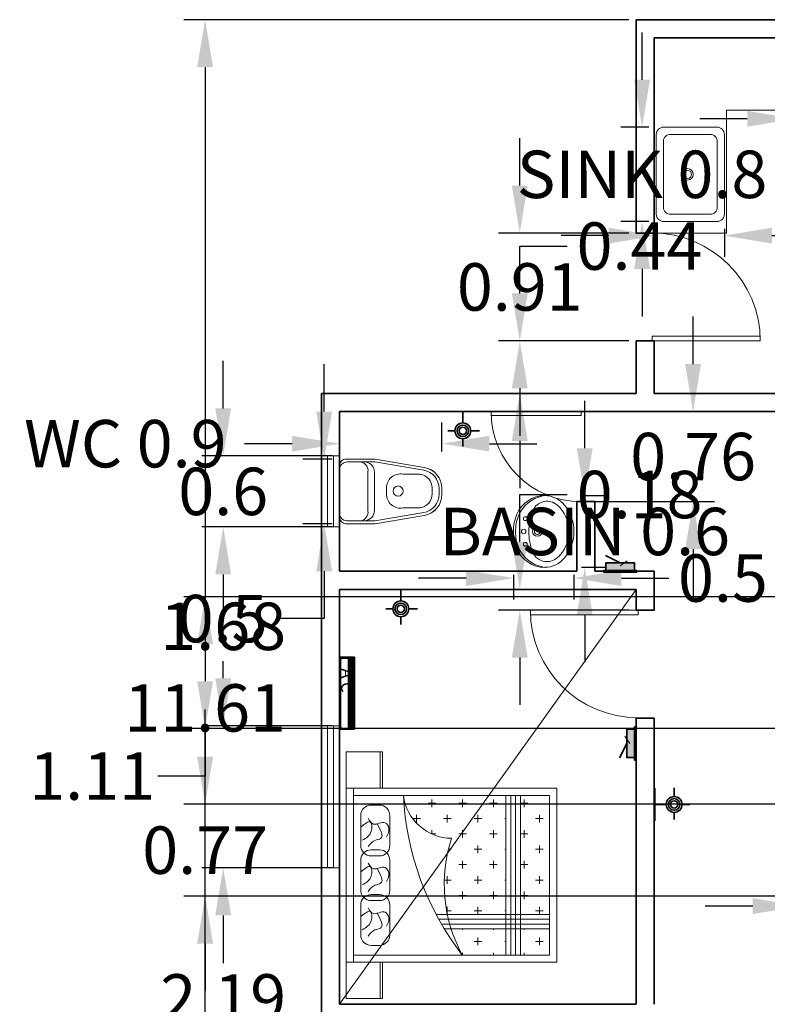
# Model space of a CAD drawing. Units: metres. Extents: x 24.2 to 58.5, y -14.5 to 15.2.
# Tile 5 of 7: x 38.9 to 45.2, y 5.2 to 13.5. Entities that reach past the tile are written whole.
import ezdxf

# ---------------------------------------------------------------- set-up
doc = ezdxf.new("R2010")
doc.units = ezdxf.units.M
doc.header["$MEASUREMENT"] = 0
for name, color, linetype, lineweight in [('A-FLOR-CASE', 163, 'Continuous', 18), ('A-FLOR-FIXT', 163, 'Continuous', 18), ('A-FURN', 150, 'Continuous', 5), ('A-GLAZ', 15, 'Continuous', 18), ('A-WALL', 7, 'Continuous', 35), ('DIMENSION', 90, 'Continuous', 18), ('DOOR', 15, 'Continuous', 18), ('E-EQPM-LAYO', 1, 'Continuous', 13), ('E-LITE', 1, 'Continuous', 18), ('E-POWR', 1, 'Continuous', 18), ('E-POWR-EQPM', 1, 'Continuous', 18), ('Elec', 1, 'Continuous', 35), ('FURN', 163, 'Continuous', 13)]:
    doc.layers.add(name, color=color, linetype=linetype, lineweight=lineweight)
doc.styles.get("Standard").update_dxf_attribs({"font": 'arial.ttf'})
doc.dimstyles.get("Standard").update_dxf_attribs({"dimtxt": 0.4, "dimasz": 0.4, "dimexe": 0.18, "dimexo": 0.0625, "dimgap": 0.09, "dimtad": 0, "dimtih": 1, "dimtoh": 1, "dimdec": 1, "dimzin": 0, "dimdsep": 46, "dimtxsty": 'Standard', "dimcen": 0.09, "dimadec": 0, "dimazin": 0, "dimtfac": 1, "dimtdec": 1, "dimtofl": 0, "dimtmove": 0, "dimatfit": 3, "dimfxl": 1, "dimtolj": 1, "dimtzin": 0, "dimarcsym": 0})

# ---------------------------------------------------------------- blocks, each defined once
blk = doc.blocks.new('*U17')
for p, q in [((0, 0), (0, -6)), ((40, 0), (40, -6))]:
    blk.add_line(p, q)
blk.add_lwpolyline([(0, 0), (0, 40), (1.75, 40), (1.75, 0)], close=True)
blk.add_arc((0, 0), 40, 0, 90)
blk = doc.blocks.new('WC')
at = {"layer": 'A-FURN'}
for p, q in [((171114.18, -56009.21), (171100.52, -56011.54)), ((171114.18, -56009.21), (171122.29, -56009.21)), ((171124.07, -56010.99), (171124.07, -56025.42)), ((171095.59, -56017.39), (171095.59, -56019.02)), ((171114.18, -56027.21), (171100.52, -56024.87)), ((171122.29, -56027.21), (171114.18, -56027.21))]:
    blk.add_line(p, q, dxfattribs=at)
for points in [[(171114.18, -56027.21), (171122.29, -56027.21, 0.414214), (171124.07, -56025.42), (171124.07, -56010.99, 0.414214), (171122.29, -56009.21), (171114.18, -56009.21), (171100.52, -56011.54, 0.365402), (171095.59, -56017.39), (171095.59, -56019.02, 0.365402), (171100.52, -56024.87)], [(171114.25, -56026.41), (171121.5, -56026.41, 0.361508), (171124.07, -56024.7), (171124.07, -56011.71, 0.375474), (171121.68, -56010), (171114.25, -56010), (171100.66, -56012.32, 0.365402), (171096.38, -56017.39), (171096.38, -56019.02, 0.365402), (171100.66, -56024.09)], [(171124.07, -56011.71), (171124.07, -56024.7, -0.361508), (171121.5, -56026.41), (171117.23, -56026.41, -0.430105), (171114.38, -56023.46), (171114.38, -56012.95, -0.411531), (171117.23, -56010), (171121.68, -56010, -0.375474)], [(171124.07, -56011.71), (171124.07, -56024.7, -0.361508), (171121.5, -56026.41), (171118.83, -56026.41, -0.480412), (171116.16, -56023.63), (171116.16, -56012.78, -0.482705), (171118.83, -56010), (171121.68, -56010, -0.375474)], [(171106.42, -56023.02, 0.46477), (171111.04, -56019.12), (171111.04, -56017.49, 0.46477), (171106.42, -56013.59), (171101.64, -56013.59, 0.365402), (171098.35, -56017.49), (171098.35, -56019.12, 0.365402), (171101.64, -56023.02)], [(171107.8, -56016.9, -1), (171107.8, -56019.71, -1)]]:
    blk.add_lwpolyline(points, format="xyb", close=True, dxfattribs=at)
for centre, radius, start, end in [((171122.29, -56010.99), 1.78, 0.0002, 90.0002), ((171101.52, -56017.39), 5.93, 99.7106, 180.0002), ((171101.52, -56019.02), 5.93, 180.0002, 260.2897), ((171122.29, -56025.42), 1.78, 270.0002, 0.0002)]:
    blk.add_arc(centre, radius, start, end, dxfattribs=at)
blk = doc.blocks.new('Basin')
at = {"layer": 'A-FURN'}
for centre, radius in [((171010.96, -56068.51), 0.593), ((171010.45, -56072.47), 0.692), ((171014.68, -56072.47), 1.48), ((171014.68, -56072.47), 0.91), ((171010.96, -56076.42), 0.593)]:
    blk.add_circle(centre, radius, dxfattribs=at)
for centre, radius, start, end in [((171018.29, -56073.43), 10.2, 262.5047, 262.5047), ((171016.96, -56070.69), 9.3, 90, 157.2856), ((171018.29, -56071.51), 10.2, 100.9967, 157.8207), ((171017.65, -56067.95), 4.81, 62.931, 159.6415), ((171016.96, -56069.3), 7.91, 39.0829, 90), ((171029.84, -56072.47), 17.8, 159.6415, 180), ((171016.96, -56069.3), 6.33, 39.0829, 62.931), ((171013.06, -56072.47), 11.35, 0, 39.0829), ((171013.06, -56072.47), 12.93, 0, 39.0829), ((171021.21, -56072.47), 13.91, 157.2856, 180), ((171021.21, -56072.47), 13.27, 158.7467, 180), ((171021.21, -56072.47), 13.91, 180, 202.7144), ((171021.21, -56072.47), 13.27, 180, 201.2533), ((171029.84, -56072.47), 17.8, 180, 200.3585), ((171013.06, -56072.47), 11.35, 320.9171, 0), ((171013.06, -56072.47), 12.93, 320.9171, 0), ((171016.96, -56074.25), 9.3, 202.7144, 270), ((171018.29, -56073.43), 10.2, 202.1793, 259.0033), ((171017.65, -56076.99), 4.81, 200.3585, 297.069), ((171016.96, -56075.63), 7.91, 270, 320.9171), ((171016.96, -56075.63), 6.33, 297.069, 320.9171)]:
    blk.add_arc(centre, radius, start, end, dxfattribs=at)
blk = doc.blocks.new('bed 1')
at = {"layer": 'FURN'}
h = blk.add_hatch(dxfattribs=at)
h.set_pattern_fill('CROSS', color=256, style=0)
h.set_pattern_definition([(0, (0, 0), (6.35, 6.35), [3.175, -9.525]), (90, (1.5875, -1.5875), (-6.35, 6.35), [3.175, -9.525])])
h.paths.add_polyline_path([(1334.16, -843.32, 0.37496), (1316.43, -863.27, 0.131129), (1284.95, -861.51), (1284.95, -885.72), (1334.16, -885.72)])
h.paths.add_polyline_path([(1278.95, -863.08, 0.048033), (1268.16, -867.67), (1268.16, -885.72), (1278.95, -885.72)])
h.paths.add_polyline_path([(1278.95, -891.72), (1268.16, -891.72), (1268.16, -903.72), (1278.95, -903.72)])
h.paths.add_polyline_path([(1334.16, -891.72), (1284.95, -891.72), (1284.95, -903.72), (1334.16, -903.72)])
for p, q in [((1265.16, -819.72), (1250.16, -819.72)), ((1250.16, -819.72), (1250.16, -834.72)), ((1337.16, -819.72), (1265.16, -819.72)), ((1265.16, -819.72), (1265.16, -906.72)), ((1337.16, -906.72), (1337.16, -819.72)), ((1337.16, -819.72), (1352.16, -819.72)), ((1352.16, -819.72), (1352.16, -834.72)), ((1337.16, -822.72), (1265.16, -822.72)), ((1268.16, -822.72), (1268.16, -903.72)), ((1334.16, -903.72), (1334.16, -822.72)), ((1250.16, -833.72), (1265.16, -833.72)), ((1352.16, -833.72), (1337.16, -833.72)), ((1250.16, -834.72), (1265.16, -834.72)), ((1352.16, -834.72), (1337.16, -834.72)), ((1282.95, -903.72), (1282.95, -857.98)), ((1284.95, -903.72), (1284.95, -856.89)), ((1278.95, -903.72), (1278.95, -860.29)), ((1280.95, -903.72), (1280.95, -859.11)), ((1334.16, -885.72), (1268.16, -885.72)), ((1334.16, -887.72), (1268.16, -887.72)), ((1334.16, -889.72), (1268.16, -889.72)), ((1334.16, -891.72), (1268.16, -891.72)), ((1268.16, -903.72), (1334.16, -903.72)), ((1265.16, -906.72), (1337.16, -906.72))]:
    blk.add_line(p, q, dxfattribs=at)
for points in [[(1288.91, -837.72), (1276.42, -837.72, -0.414214), (1272.16, -833.47), (1272.16, -829.98, -0.414214), (1276.42, -825.72), (1288.91, -825.72, -0.414214), (1293.16, -829.98), (1293.16, -833.47, -0.414214)], [(1307.41, -837.72), (1294.92, -837.72, -0.414214), (1290.66, -833.47), (1290.66, -829.98, -0.414214), (1294.92, -825.72), (1307.41, -825.72, -0.414214), (1311.66, -829.98), (1311.66, -833.47, -0.414214)], [(1325.91, -837.72), (1313.42, -837.72, -0.414214), (1309.16, -833.47), (1309.16, -829.98, -0.414214), (1313.42, -825.72), (1325.91, -825.72, -0.414214), (1330.16, -829.98), (1330.16, -833.47, -0.414214)], [(1334.16, -843.32, 0.151933), (1268.16, -867.67), (1268.16, -867.67, -0.20661), (1316.43, -863.27), (1316.43, -863.27, -0.37496)]]:
    blk.add_lwpolyline(points, format="xyb", close=True, dxfattribs=at)
for points, knots in [([(1278.62, -826.37), (1279.52, -827.92), (1281.07, -830.61), (1287.77, -830.3), (1285.41, -827.44), (1284.17, -825.93)], [0, 0, 0, 0, 4.23607, 7.317462, 10.761159, 10.761159, 10.761159, 10.761159]), ([(1297.12, -826.37), (1298.02, -827.92), (1299.57, -830.61), (1306.27, -830.3), (1303.91, -827.44), (1302.67, -825.93)], [0, 0, 0, 0, 4.23607, 7.317462, 10.761159, 10.761159, 10.761159, 10.761159]), ([(1315.62, -826.37), (1316.52, -827.92), (1318.07, -830.61), (1324.77, -830.3), (1322.41, -827.44), (1321.17, -825.93)], [0, 0, 0, 0, 4.23607, 7.317462, 10.761159, 10.761159, 10.761159, 10.761159]), ([(1275.98, -828.74), (1277, -829.54), (1278.71, -830.85), (1279.22, -835.95), (1282.92, -833.91), (1285.58, -832.44)], [0, 0, 0, 0, 3.079719, 5.108686, 10.317752, 10.317752, 10.317752, 10.317752]), ([(1287.7, -828.74), (1286.63, -829.38), (1283.96, -830.98), (1287.28, -835.52), (1283.18, -838.02), (1281.17, -836.99), (1280.03, -836.4)], [0, 0, 0, 0, 2.624379, 6.568207, 8.823918, 11.783788, 11.783788, 11.783788, 11.783788]), ([(1294.48, -828.74), (1295.5, -829.54), (1297.21, -830.85), (1297.72, -835.95), (1301.42, -833.91), (1304.08, -832.44)], [0, 0, 0, 0, 3.079719, 5.108686, 10.317752, 10.317752, 10.317752, 10.317752]), ([(1306.2, -828.74), (1305.13, -829.38), (1302.46, -830.98), (1305.78, -835.52), (1301.68, -838.02), (1299.67, -836.99), (1298.53, -836.4)], [0, 0, 0, 0, 2.624379, 6.568207, 8.823918, 11.783788, 11.783788, 11.783788, 11.783788]), ([(1312.98, -828.74), (1314, -829.54), (1315.71, -830.85), (1316.22, -835.95), (1319.92, -833.91), (1322.58, -832.44)], [0, 0, 0, 0, 3.079719, 5.108686, 10.317752, 10.317752, 10.317752, 10.317752]), ([(1324.7, -828.74), (1323.63, -829.38), (1320.96, -830.98), (1324.28, -835.52), (1320.18, -838.02), (1318.17, -836.99), (1317.03, -836.4)], [0, 0, 0, 0, 2.624379, 6.568207, 8.823918, 11.783788, 11.783788, 11.783788, 11.783788])]:
    blk.add_open_spline(points, degree=3, knots=knots, dxfattribs=at)
blk = doc.blocks.new('SINK')
at = {"layer": 'A-FURN'}
for points in [[(42.3016, 12.7524), (42.9757, 12.7524, -0.414214), (43.0363, 12.6917), (43.0363, 12.2383, -0.414214), (42.9757, 12.1776), (42.3016, 12.1776, -0.414214), (42.2409, 12.2383), (42.2409, 12.6917, -0.414214)], [(42.3622, 12.6917), (42.915, 12.6917, -0.414214), (42.9757, 12.6311), (42.9757, 12.2989, -0.414214), (42.915, 12.2383), (42.3622, 12.2383, -0.414214), (42.3016, 12.2989), (42.3016, 12.6311, -0.414214)]]:
    blk.add_lwpolyline(points, format="xyb", close=True, dxfattribs=at)
for radius in [0.0481, 0.0337]:
    blk.add_circle((42.6387, 12.4417), radius, dxfattribs=at)
blk = doc.blocks.new('splight')
at = {"layer": 'Elec'}
for p, q in [((4618.17, 527.16), (4627.57, 527.16)), ((4622.87, 527.16), (4622.87, 523.87)), ((4620.58, 521.58), (4618.05, 521.58)), ((4625.16, 521.58), (4627.23, 521.58)), ((4622.87, 519.28), (4622.87, 517.03))]:
    blk.add_line(p, q, dxfattribs=at)
for radius in [2.29, 1.67, 1.04]:
    blk.add_circle((4622.87, 521.58), radius, dxfattribs=at)
blk = doc.blocks.new('ac')
at = {"layer": 'Elec'}
for p, q in [((12718.34, -53.78), (12674.36, -53.78)), ((12674.36, -63.02), (12674.36, -53.78)), ((12675.81, -57.52), (12675.81, -53.78)), ((12717.03, -57.52), (12717.03, -53.78)), ((12718.34, -63.02), (12718.34, -53.78)), ((12674.89, -57.52), (12717.81, -57.52)), ((12717.03, -54.85), (12675.81, -54.85)), ((12717.03, -56.21), (12675.81, -56.21)), ((12718.34, -63.02), (12674.36, -63.02))]:
    blk.add_line(p, q, dxfattribs=at)
at = {"layer": 'Elec', "ltscale": 0.1}
for p, q in [((12674.89, -61.49), (12674.89, -53.78)), ((12717.81, -61.49), (12717.81, -53.78)), ((12717.03, -54.36), (12675.81, -54.36)), ((12717.03, -55.66), (12675.81, -55.66)), ((12717.03, -56.84), (12675.81, -56.84)), ((12716.81, -62.49), (12675.89, -62.49))]:
    blk.add_line(p, q, dxfattribs=at)
at = {"layer": 'Elec'}
for centre, start, end in [((12675.89, -61.49), 180, 270), ((12716.81, -61.49), 270, 0)]:
    blk.add_arc(centre, 1, start, end, dxfattribs=at)
blk = doc.blocks.new('WINDOW-1200')
for p, q in [((0.1529, 1.1998), (0.0005, 1.1998)), ((0.0513, -0.0002), (0.0513, 1.1998)), ((0.1021, -0.0002), (0.1021, 1.1998)), ((0.1529, -0.0002), (0.0005, -0.0002))]:
    blk.add_line(p, q)
blk = doc.blocks.new('elec box')
at = {"layer": 'Elec'}
blk.add_hatch(color=256, dxfattribs=at).paths.add_polyline_path([(3828.23, 599.29), (3828.23, 594.79), (3844.73, 594.79), (3844.73, 599.29)])
for p, q in [((3836.48, 599.29), (3828.07, 603.45)), ((3846.1, 594.79), (3826.83, 594.79)), ((3826.83, 594.79), (3826.83, 593.89)), ((3826.83, 593.89), (3846.1, 593.89)), ((3846.1, 593.89), (3846.1, 594.79))]:
    blk.add_line(p, q, dxfattribs=at)
blk.add_lwpolyline([(3828.23, 594.79), (3828.23, 599.29), (3844.73, 599.29), (3844.73, 594.79), (3828.23, 594.79)], dxfattribs=at)
blk = doc.blocks.new('SWITCHBOARD-ONE-WAY')
blk.add_line((0.1401, 0.0521), (0.201, 0.0944))
at = {"xscale": 0.0145668999005024, "yscale": 0.0145668999005024, "zscale": 0.0145668999005024}
blk.add_blockref('elec box', (-55.7455, -8.6514), dxfattribs=at)
blk = doc.blocks.new('*D71')
at = {"layer": 'Defpoints', "color": 0, "transparency": 16777216}
for p in [(41.5755, 9.9299), (41.5755, 9.8003), (42.4392, 9.8003)]:
    blk.add_point(p, dxfattribs=at)
at = {"layer": 'DIMENSION', "color": 0, "lineweight": -2, "transparency": 16777216}
for p, q in [((41.5755, 9.8628), (41.5755, 10.1099)), ((42.4392, 9.8628), (42.4392, 10.1099)), ((41.1755, 9.9299), (40.7755, 9.9299)), ((42.8392, 9.9299), (43.2392, 9.9299))]:
    blk.add_line(p, q, dxfattribs=at)
at = {"layer": 'DIMENSION', "color": 0, "transparency": 16777216}
for points in [[(41.1755, 9.9966), (41.1755, 9.8632), (41.5755, 9.9299)], [(42.8392, 9.9966), (42.8392, 9.8632), (42.4392, 9.9299)]]:
    blk.add_solid(points, dxfattribs=at)
at = {"layer": 'DIMENSION', "color": 0, "transparency": 16777216, "insert": (39.7697, 9.9299), "char_height": 0.4, "attachment_point": 5}
blk.add_mtext('\\A1;WC 0.9', dxfattribs=at)
blk = doc.blocks.new('*D72')
at = {"layer": 'Defpoints', "color": 0, "transparency": 16777216}
for p in [(41.5755, 9.8003), (41.4459, 9.2545), (41.5755, 9.2545)]:
    blk.add_point(p, dxfattribs=at)
at = {"layer": 'DIMENSION', "color": 0, "lineweight": -2, "transparency": 16777216}
for p, q in [((41.4459, 10.2003), (41.4459, 10.6003)), ((41.513, 9.8003), (41.2659, 9.8003)), ((41.513, 9.2545), (41.2659, 9.2545)), ((41.4459, 8.8545), (41.4459, 8.4545)), ((41.4459, 8.4545), (41.0459, 8.4545))]:
    blk.add_line(p, q, dxfattribs=at)
at = {"layer": 'DIMENSION', "color": 0, "transparency": 16777216}
for points in [[(41.3793, 10.2003), (41.5126, 10.2003), (41.4459, 9.8003)], [(41.3793, 8.8545), (41.5126, 8.8545), (41.4459, 9.2545)]]:
    blk.add_solid(points, dxfattribs=at)
at = {"layer": 'DIMENSION', "color": 0, "transparency": 16777216, "insert": (40.5903, 8.4545), "char_height": 0.4, "attachment_point": 5}
blk.add_mtext('\\A1;0.5', dxfattribs=at)
blk = doc.blocks.new('*D73')
at = {"layer": 'Defpoints', "color": 0, "transparency": 16777216}
for p in [(43.5517, 9.4916), (43.6424, 9.4916), (43.5517, 8.8871)]:
    blk.add_point(p, dxfattribs=at)
at = {"layer": 'DIMENSION', "color": 0, "lineweight": -2, "transparency": 16777216}
for p, q in [((43.6424, 9.8916), (43.6424, 10.2916)), ((43.6142, 9.4916), (43.8224, 9.4916)), ((43.6142, 8.8871), (43.8224, 8.8871)), ((43.6424, 8.4871), (43.6424, 8.0871))]:
    blk.add_line(p, q, dxfattribs=at)
at = {"layer": 'DIMENSION', "color": 0, "transparency": 16777216}
for points in [[(43.5758, 9.8916), (43.7091, 9.8916), (43.6424, 9.4916)], [(43.5758, 8.4871), (43.7091, 8.4871), (43.6424, 8.8871)]]:
    blk.add_solid(points, dxfattribs=at)
at = {"layer": 'DIMENSION', "color": 0, "transparency": 16777216, "insert": (43.6424, 9.1893), "char_height": 0.4, "attachment_point": 5}
blk.add_mtext('\\A1;BASIN 0.6', dxfattribs=at)
blk = doc.blocks.new('*D74')
at = {"layer": 'Defpoints', "color": 0, "transparency": 16777216}
for p in [(43.0417, 8.8871), (43.5517, 8.8871), (43.5517, 8.7964)]:
    blk.add_point(p, dxfattribs=at)
at = {"layer": 'DIMENSION', "color": 0, "lineweight": -2, "transparency": 16777216}
for p, q in [((43.0417, 8.8246), (43.0417, 8.6164)), ((43.5517, 8.8246), (43.5517, 8.6164)), ((42.6417, 8.7964), (42.2417, 8.7964)), ((43.9517, 8.7964), (44.3517, 8.7964))]:
    blk.add_line(p, q, dxfattribs=at)
at = {"layer": 'DIMENSION', "color": 0, "transparency": 16777216}
for points in [[(42.6417, 8.863), (42.6417, 8.7297), (43.0417, 8.7964)], [(43.9517, 8.863), (43.9517, 8.7297), (43.5517, 8.7964)]]:
    blk.add_solid(points, dxfattribs=at)
at = {"layer": 'DIMENSION', "color": 0, "transparency": 16777216, "insert": (44.8074, 8.7964), "char_height": 0.4, "attachment_point": 5}
blk.add_mtext('\\A1;0.5', dxfattribs=at)
blk = doc.blocks.new('*D77')
at = {"layer": 'Defpoints', "color": 0, "transparency": 16777216}
for p in [(45.4122, 12.817), (46.3908, 12.817), (46.3908, 12.6703)]:
    blk.add_point(p, dxfattribs=at)
at = {"layer": 'DIMENSION', "color": 0, "lineweight": -2, "transparency": 16777216}
for p, q in [((45.4122, 12.7545), (45.4122, 12.4903)), ((46.3908, 12.7545), (46.3908, 12.4903)), ((45.0122, 12.6703), (44.6122, 12.6703)), ((46.7908, 12.6703), (47.1908, 12.6703))]:
    blk.add_line(p, q, dxfattribs=at)
at = {"layer": 'DIMENSION', "color": 0, "transparency": 16777216}
for points in [[(45.0122, 12.7369), (45.0122, 12.6036), (45.4122, 12.6703)], [(46.7908, 12.7369), (46.7908, 12.6036), (46.3908, 12.6703)]]:
    blk.add_solid(points, dxfattribs=at)
at = {"layer": 'DIMENSION', "color": 0, "transparency": 16777216, "insert": (48.3165, 12.6703), "char_height": 0.4, "attachment_point": 5}
blk.add_mtext('\\A1;HOB 1.0', dxfattribs=at)
blk = doc.blocks.new('*D79')
at = {"layer": 'Defpoints', "color": 0, "transparency": 16777216}
for p in [(44.2452, 12.5993), (44.1259, 11.8039), (44.2452, 11.8039)]:
    blk.add_point(p, dxfattribs=at)
at = {"layer": 'DIMENSION', "color": 0, "lineweight": -2, "transparency": 16777216}
for p, q in [((44.1259, 12.9993), (44.1259, 13.3993)), ((44.1827, 12.5993), (43.9459, 12.5993)), ((44.1827, 11.8039), (43.9459, 11.8039)), ((44.1259, 11.4039), (44.1259, 11.0039))]:
    blk.add_line(p, q, dxfattribs=at)
at = {"layer": 'DIMENSION', "color": 0, "transparency": 16777216}
for points in [[(44.0592, 12.9993), (44.1926, 12.9993), (44.1259, 12.5993)], [(44.0592, 11.4039), (44.1926, 11.4039), (44.1259, 11.8039)]]:
    blk.add_solid(points, dxfattribs=at)
at = {"layer": 'DIMENSION', "color": 0, "transparency": 16777216, "insert": (44.1259, 12.2016), "char_height": 0.4, "attachment_point": 5}
blk.add_mtext('\\A1;SINK 0.8', dxfattribs=at)
blk = doc.blocks.new('*D80')
at = {"layer": 'Defpoints', "color": 0, "transparency": 16777216}
for p in [(44.2452, 11.8039), (44.82, 11.8039), (44.82, 11.6846)]:
    blk.add_point(p, dxfattribs=at)
at = {"layer": 'DIMENSION', "color": 0, "lineweight": -2, "transparency": 16777216}
for p, q in [((44.2452, 11.7414), (44.2452, 11.5046)), ((44.82, 11.7414), (44.82, 11.5046)), ((43.8452, 11.6846), (43.4452, 11.6846)), ((45.22, 11.6846), (45.62, 11.6846))]:
    blk.add_line(p, q, dxfattribs=at)
at = {"layer": 'DIMENSION', "color": 0, "transparency": 16777216}
for points in [[(43.8452, 11.7513), (43.8452, 11.6179), (44.2452, 11.6846)], [(45.22, 11.7513), (45.22, 11.6179), (44.82, 11.6846)]]:
    blk.add_solid(points, dxfattribs=at)
at = {"layer": 'DIMENSION', "color": 0, "transparency": 16777216, "insert": (46.074, 11.6846), "char_height": 0.4, "attachment_point": 5}
blk.add_mtext('\\A1;0.6', dxfattribs=at)
blk = doc.blocks.new('*D108')
at = {"layer": 'Defpoints', "color": 0, "transparency": 16777216}
for p in [(40.4426, 13.506), (44.0755, 13.506), (41.4231, 1.8964)]:
    blk.add_point(p, dxfattribs=at)
at = {"layer": 'DIMENSION', "color": 0, "lineweight": -2, "transparency": 16777216}
for p, q in [((44.013, 13.506), (40.2626, 13.506)), ((40.4426, 13.106), (40.4426, 7.9955)), ((40.4426, 2.2964), (40.4426, 7.407)), ((41.3606, 1.8964), (40.2626, 1.8964))]:
    blk.add_line(p, q, dxfattribs=at)
at = {"layer": 'DIMENSION', "color": 0, "transparency": 16777216}
for points in [[(40.3759, 13.106), (40.5092, 13.106), (40.4426, 13.506)], [(40.3759, 2.2964), (40.5092, 2.2964), (40.4426, 1.8964)]]:
    blk.add_solid(points, dxfattribs=at)
at = {"layer": 'DIMENSION', "color": 0, "transparency": 16777216, "insert": (40.4426, 7.7012), "char_height": 0.4, "attachment_point": 5}
blk.add_mtext('\\A1;11.61', dxfattribs=at)
blk = doc.blocks.new('*D110')
at = {"layer": 'Defpoints', "color": 0, "transparency": 16777216}
for p in [(40.595, 6.3512), (41.5755, 6.3512), (41.5755, 4.1588)]:
    blk.add_point(p, dxfattribs=at)
at = {"layer": 'DIMENSION', "color": 0, "lineweight": -2, "transparency": 16777216}
for p, q in [((41.513, 6.3512), (40.415, 6.3512)), ((40.595, 5.9512), (40.595, 5.5493)), ((40.595, 4.5588), (40.595, 4.9608)), ((41.513, 4.1588), (40.415, 4.1588))]:
    blk.add_line(p, q, dxfattribs=at)
at = {"layer": 'DIMENSION', "color": 0, "transparency": 16777216}
for points in [[(40.5283, 5.9512), (40.6616, 5.9512), (40.595, 6.3512)], [(40.5283, 4.5588), (40.6616, 4.5588), (40.595, 4.1588)]]:
    blk.add_solid(points, dxfattribs=at)
at = {"layer": 'DIMENSION', "color": 0, "transparency": 16777216, "insert": (40.595, 5.255), "char_height": 0.4, "attachment_point": 5}
blk.add_mtext('\\A1;2.19', dxfattribs=at)
blk = doc.blocks.new('*D111')
at = {"layer": 'Defpoints', "color": 0, "transparency": 16777216}
for p in [(40.595, 9.2274), (41.5755, 9.2274), (41.5755, 7.5512)]:
    blk.add_point(p, dxfattribs=at)
at = {"layer": 'DIMENSION', "color": 0, "lineweight": -2, "transparency": 16777216}
for p, q in [((41.513, 9.2274), (40.415, 9.2274)), ((40.595, 8.8274), (40.595, 8.6836)), ((40.595, 7.9512), (40.595, 8.0951)), ((41.513, 7.5512), (40.415, 7.5512))]:
    blk.add_line(p, q, dxfattribs=at)
at = {"layer": 'DIMENSION', "color": 0, "transparency": 16777216}
for points in [[(40.5283, 8.8274), (40.6617, 8.8274), (40.595, 9.2274)], [(40.5283, 7.9512), (40.6617, 7.9512), (40.595, 7.5512)]]:
    blk.add_solid(points, dxfattribs=at)
at = {"layer": 'DIMENSION', "color": 0, "transparency": 16777216, "insert": (40.595, 8.3893), "char_height": 0.4, "attachment_point": 5}
blk.add_mtext('\\A1;1.68', dxfattribs=at)
blk = doc.blocks.new('*D112')
at = {"layer": 'Defpoints', "color": 0, "transparency": 16777216}
for p in [(40.595, 9.8274), (41.5755, 9.8274), (41.5755, 9.2274)]:
    blk.add_point(p, dxfattribs=at)
at = {"layer": 'DIMENSION', "color": 0, "lineweight": -2, "transparency": 16777216}
for p, q in [((40.595, 10.2274), (40.5949, 10.6274)), ((41.513, 9.8274), (40.415, 9.8274)), ((41.513, 9.2274), (40.415, 9.2274)), ((40.595, 8.8274), (40.595, 8.4274))]:
    blk.add_line(p, q, dxfattribs=at)
at = {"layer": 'DIMENSION', "color": 0, "transparency": 16777216}
for points in [[(40.6616, 10.2274), (40.5283, 10.2274), (40.595, 9.8274)], [(40.6617, 8.8274), (40.5283, 8.8274), (40.595, 9.2274)]]:
    blk.add_solid(points, dxfattribs=at)
at = {"layer": 'DIMENSION', "color": 0, "transparency": 16777216, "insert": (40.595, 9.5274), "char_height": 0.4, "attachment_point": 5}
blk.add_mtext('\\A1;0.6', dxfattribs=at)
blk = doc.blocks.new('*D120')
at = {"layer": 'Defpoints', "color": 0, "transparency": 16777216}
for p in [(49.2027, 6.8888), (40.4426, 6.114), (49.1166, 6.114)]:
    blk.add_point(p, dxfattribs=at)
at = {"layer": 'DIMENSION', "color": 0, "lineweight": -2, "transparency": 16777216}
for p, q in [((40.4426, 7.2888), (40.4426, 7.6888)), ((49.1402, 6.8888), (40.2626, 6.8888)), ((49.0541, 6.114), (40.2626, 6.114)), ((40.4426, 5.714), (40.4426, 5.314))]:
    blk.add_line(p, q, dxfattribs=at)
at = {"layer": 'DIMENSION', "color": 0, "transparency": 16777216}
for points in [[(40.3759, 7.2888), (40.5092, 7.2888), (40.4426, 6.8888)], [(40.3759, 5.714), (40.5092, 5.714), (40.4426, 6.114)]]:
    blk.add_solid(points, dxfattribs=at)
at = {"layer": 'DIMENSION', "color": 0, "transparency": 16777216, "insert": (40.4426, 6.5014), "char_height": 0.4, "attachment_point": 5}
blk.add_mtext('\\A1;0.77', dxfattribs=at)
blk = doc.blocks.new('*D122')
at = {"layer": 'Defpoints', "color": 0, "transparency": 16777216}
for p in [(49.5878, 8.6391), (40.4426, 7.5263), (49.5878, 7.5263)]:
    blk.add_point(p, dxfattribs=at)
at = {"layer": 'DIMENSION', "color": 0, "lineweight": -2, "transparency": 16777216}
for p, q in [((49.5253, 8.6391), (40.2626, 8.6391)), ((40.4426, 8.2391), (40.4426, 7.9263)), ((49.5253, 7.5263), (40.2626, 7.5263)), ((40.4426, 7.5263), (40.4426, 7.1263)), ((40.4426, 7.1263), (40.0426, 7.1263))]:
    blk.add_line(p, q, dxfattribs=at)
at = {"layer": 'DIMENSION', "color": 0, "transparency": 16777216}
for points in [[(40.3759, 8.2391), (40.5092, 8.2391), (40.4426, 8.6391)], [(40.3759, 7.9263), (40.5092, 7.9263), (40.4426, 7.5263)]]:
    blk.add_solid(points, dxfattribs=at)
at = {"layer": 'DIMENSION', "color": 0, "transparency": 16777216, "insert": (39.4905, 7.1263), "char_height": 0.4, "attachment_point": 5}
blk.add_mtext('\\A1;1.11', dxfattribs=at)
blk = doc.blocks.new('*D123')
at = {"layer": 'Defpoints', "color": 0, "transparency": 16777216}
for p in [(43.095, 10.7967), (44.0755, 10.7967), (44.0755, 10.3536)]:
    blk.add_point(p, dxfattribs=at)
at = {"layer": 'DIMENSION', "color": 0, "lineweight": -2, "transparency": 16777216}
for p, q in [((43.095, 11.1967), (43.095, 11.5967)), ((43.095, 11.5967), (43.495, 11.5967)), ((44.013, 10.7967), (42.915, 10.7967)), ((44.013, 10.3536), (42.915, 10.3536)), ((43.095, 9.9536), (43.095, 9.5536))]:
    blk.add_line(p, q, dxfattribs=at)
at = {"layer": 'DIMENSION', "color": 0, "transparency": 16777216}
for points in [[(43.0283, 11.1967), (43.1616, 11.1967), (43.095, 10.7967)], [(43.0283, 9.9536), (43.1616, 9.9536), (43.095, 10.3536)]]:
    blk.add_solid(points, dxfattribs=at)
at = {"layer": 'DIMENSION', "color": 0, "transparency": 16777216, "insert": (44.1037, 11.5967), "char_height": 0.4, "attachment_point": 5}
blk.add_mtext('\\A1;0.44', dxfattribs=at)
blk = doc.blocks.new('*D124')
at = {"layer": 'Defpoints', "color": 0, "transparency": 16777216}
for p in [(43.095, 8.7012), (44.0755, 8.7012), (44.0755, 8.5258)]:
    blk.add_point(p, dxfattribs=at)
at = {"layer": 'DIMENSION', "color": 0, "lineweight": -2, "transparency": 16777216}
for p, q in [((43.095, 9.1012), (43.095, 9.5012)), ((43.095, 9.5012), (43.495, 9.5012)), ((44.013, 8.7012), (42.915, 8.7012)), ((44.013, 8.5258), (42.915, 8.5258)), ((43.095, 8.1258), (43.095, 7.7258))]:
    blk.add_line(p, q, dxfattribs=at)
at = {"layer": 'DIMENSION', "color": 0, "transparency": 16777216}
for points in [[(43.0283, 9.1012), (43.1616, 9.1012), (43.095, 8.7012)], [(43.0283, 8.1258), (43.1616, 8.1258), (43.095, 8.5258)]]:
    blk.add_solid(points, dxfattribs=at)
at = {"layer": 'DIMENSION', "color": 0, "transparency": 16777216, "insert": (44.1049, 9.5012), "char_height": 0.4, "attachment_point": 5}
blk.add_mtext('\\A1;0.18', dxfattribs=at)
blk = doc.blocks.new('*D125')
at = {"layer": 'Defpoints', "color": 0, "transparency": 16777216}
for p in [(45.5755, 6.0293), (45.4589, 5.0488), (45.5755, 5.0488)]:
    blk.add_point(p, dxfattribs=at)
at = {"layer": 'DIMENSION', "color": 0, "lineweight": -2, "transparency": 16777216}
for p, q in [((45.4589, 5.1113), (45.4589, 6.2093)), ((45.5755, 5.1113), (45.5755, 6.2093)), ((45.0589, 6.0293), (44.6589, 6.0293)), ((45.9755, 6.0293), (46.3755, 6.0293))]:
    blk.add_line(p, q, dxfattribs=at)
at = {"layer": 'DIMENSION', "color": 0, "transparency": 16777216}
for points in [[(45.0589, 6.096), (45.0589, 5.9627), (45.4589, 6.0293)], [(45.9755, 6.096), (45.9755, 5.9627), (45.5755, 6.0293)]]:
    blk.add_solid(points, dxfattribs=at)
at = {"layer": 'DIMENSION', "color": 0, "transparency": 16777216, "insert": (46.9829, 6.0293), "char_height": 0.4, "attachment_point": 5}
blk.add_mtext('\\A1;0.12', dxfattribs=at)
blk = doc.blocks.new('*D126')
at = {"layer": 'Defpoints', "color": 0, "transparency": 16777216}
for p in [(43.095, 11.7068), (44.0755, 11.7068), (44.0755, 10.7967)]:
    blk.add_point(p, dxfattribs=at)
at = {"layer": 'DIMENSION', "color": 0, "lineweight": -2, "transparency": 16777216}
for p, q in [((43.095, 12.1068), (43.095, 12.5068)), ((44.013, 11.7068), (42.915, 11.7068)), ((44.013, 10.7967), (42.915, 10.7967)), ((43.095, 10.3967), (43.095, 9.9967))]:
    blk.add_line(p, q, dxfattribs=at)
at = {"layer": 'DIMENSION', "color": 0, "transparency": 16777216}
for points in [[(43.0283, 12.1068), (43.1616, 12.1068), (43.095, 11.7068)], [(43.0283, 10.3967), (43.1616, 10.3967), (43.095, 10.7967)]]:
    blk.add_solid(points, dxfattribs=at)
at = {"layer": 'DIMENSION', "color": 0, "transparency": 16777216, "insert": (43.095, 11.2518), "char_height": 0.4, "attachment_point": 5}
blk.add_mtext('\\A1;0.91', dxfattribs=at)
blk = doc.blocks.new('*D127')
at = {"layer": 'Defpoints', "color": 0, "transparency": 16777216}
for p in [(43.5755, 10.2012), (43.5755, 9.4412), (44.556, 9.4412)]:
    blk.add_point(p, dxfattribs=at)
at = {"layer": 'DIMENSION', "color": 0, "lineweight": -2, "transparency": 16777216}
for p, q in [((44.556, 10.6012), (44.556, 11.0012)), ((43.638, 10.2012), (44.736, 10.2012)), ((43.638, 9.4412), (44.736, 9.4412)), ((44.556, 9.0412), (44.556, 8.6412))]:
    blk.add_line(p, q, dxfattribs=at)
at = {"layer": 'DIMENSION', "color": 0, "transparency": 16777216}
for points in [[(44.4893, 10.6012), (44.6226, 10.6012), (44.556, 10.2012)], [(44.4893, 9.0412), (44.6226, 9.0412), (44.556, 9.4412)]]:
    blk.add_solid(points, dxfattribs=at)
at = {"layer": 'DIMENSION', "color": 0, "transparency": 16777216, "insert": (44.556, 9.8212), "char_height": 0.4, "attachment_point": 5}
blk.add_mtext('\\A1;0.76', dxfattribs=at)

msp = doc.modelspace()

# ---------------------------------------------------------------- linework, layer by layer
at = {"layer": 'A-FLOR-CASE'}
for p, q in [((44.8379, 12.7436), (47.0177, 12.7436)), ((44.8379, 11.7067), (44.8379, 12.7436)), ((44.8379, 11.7067), (44.212, 11.7068))]:
    msp.add_line(p, q, dxfattribs=at)
at = {"layer": 'A-GLAZ'}
for p, q in [((41.5755, 9.8274), (41.4231, 9.8274)), ((41.4739, 9.2274), (41.4739, 9.8274)), ((41.5247, 9.2274), (41.5247, 9.8274)), ((41.5755, 9.2274), (41.4231, 9.2274))]:
    msp.add_line(p, q, dxfattribs=at)
at = {"layer": 'A-WALL'}
for p, q in [((44.0755, 13.506), (48.2279, 13.506)), ((44.0755, 11.7067), (44.0755, 13.506)), ((44.2279, 13.3536), (48.0755, 13.3536)), ((44.2279, 11.7067), (44.2279, 13.3536)), ((44.2279, 11.7067), (44.0755, 11.7067)), ((44.0755, 10.3536), (44.0755, 10.7967)), ((44.2279, 10.7967), (44.0755, 10.7967)), ((44.2279, 10.3536), (44.2279, 10.7967)), ((41.4231, 10.3536), (44.0755, 10.3536)), ((41.4231, 1.8964), (41.4231, 10.3536)), ((44.2279, 10.3536), (46.3865, 10.3536)), ((41.5755, 10.2012), (43.5755, 10.2012)), ((41.5755, 8.8536), (41.5755, 10.2012)), ((43.7279, 10.2012), (43.5755, 10.2012)), ((43.7279, 10.2012), (46.3865, 10.2012)), ((43.5755, 8.8536), (43.5755, 9.4412)), ((43.7279, 9.4412), (43.5755, 9.4412)), ((43.7279, 8.8536), (43.7279, 9.4412)), ((41.5755, 8.8536), (43.5755, 8.8536)), ((43.7279, 8.8536), (44.2279, 8.8536)), ((44.2279, 8.5258), (44.2279, 8.8536)), ((41.5755, 8.7012), (44.0755, 8.7012)), ((41.5755, 5.2012), (41.5755, 8.7012)), ((44.0755, 8.5258), (44.0755, 8.7012)), ((44.0755, 8.5258), (44.2279, 8.5258)), ((44.0755, 5.2012), (44.0755, 7.6158)), ((44.0755, 7.6158), (44.2279, 7.6158)), ((44.2279, 5.2012), (44.2279, 7.6158)), ((41.5755, 5.2012), (44.0755, 5.2012))]:
    msp.add_line(p, q, dxfattribs=at)
at = {"layer": 'E-EQPM-LAYO'}
msp.add_line((41.5755, 5.2012), (44.0755, 8.7012), dxfattribs=at)

# ---------------------------------------------------------------- block references
at = {"layer": 'A-FLOR-FIXT', "rotation": 270}
msp.add_blockref('SINK', (32.0676, 54.8402), dxfattribs=at)
at = {"layer": 'A-FLOR-FIXT', "xscale": 0.0303227481289544, "yscale": 0.0303227481289544, "zscale": 0.0303227481289544, "rotation": 180}
msp.add_blockref('WC', (5230.5277, -1689.0985), dxfattribs=at)
at = {"layer": 'A-FLOR-FIXT', "ltscale": 0.05, "xscale": 0.0272904733167649, "yscale": 0.0272904733167649, "zscale": 0.0272904733167649}
msp.add_blockref('Basin', (-4623.8286, 1539.4335), dxfattribs=at)
at = {"layer": 'A-GLAZ'}
msp.add_blockref('WINDOW-1200', (41.4226, 6.3514), dxfattribs=at)
at = {"layer": 'DOOR'}
for p, xscale, yscale, zscale, rotation in [((44.212, 10.7967), -0.0227525982190626, 0.0227525982190626, 0.0227525982190626, 270), ((43.6137, 10.2012), -0.0190267575646439, 0.0190267575646439, 0.0190267575646439, 90), ((44.0918, 8.5258), -0.0226837224149936, 0.0226837224149936, 0.0226837224149936, 90)]:
    msp.add_blockref('*U17', p, dxfattribs=dict(at, xscale=xscale, yscale=yscale, zscale=zscale, rotation=rotation))
at = {"layer": 'E-LITE', "xscale": -0.0291629336008972, "yscale": 0.0291629336008972, "zscale": 0.0291629336007624}
for p, rotation in [((177.4315, -5.1723), 359.9999999999997), ((176.9083, -6.6742), 359.9999999999997), ((59.6075, 141.7036), 89.99999999999976)]:
    msp.add_blockref('splight', p, dxfattribs=dict(at, rotation=rotation))
at = {"layer": 'E-POWR'}
msp.add_blockref('SWITCHBOARD-ONE-WAY', (43.8005, 8.8468), dxfattribs=at)
at = {"layer": 'E-POWR', "rotation": 89.99999999999886}
msp.add_blockref('SWITCHBOARD-ONE-WAY', (44.0752, 7.2616), dxfattribs=at)
at = {"layer": 'E-POWR-EQPM', "xscale": 0.0137983327653967, "yscale": 0.0137983327653967, "zscale": 0.0137983327653967, "rotation": 270}
msp.add_blockref('ac', (42.445, 183.0129), dxfattribs=at)
at = {"layer": 'FURN', "xscale": 0.0203972636680773, "yscale": 0.0203972636680773, "zscale": 0.0203972636680773, "rotation": 90}
msp.add_blockref('bed 1', (24.912, -20.2501), dxfattribs=at)

# ---------------------------------------------------------------- texts
at = {"layer": 'E-POWR-EQPM'}
msp.add_text(' A C', height=0.10197, rotation=270, dxfattribs=at).set_placement((41.5897, 8.0654))

# ---------------------------------------------------------------- dimensions: what is measured, and where the dimension line sits
at = {"layer": 'DIMENSION'}
for base, p1, p2, angle, override, picture, middle in [((40.4426, 13.506), (41.4231, 1.8964), (44.0755, 13.506), 90, {"dimdec": 2, "dimlfac": 1, "dimrnd": 0, "dimzin": 0, "dimdsep": 46, "dimlunit": 2}, '*D108', (40.4426, 7.7012)), ((43.095, 11.7068), (44.0755, 10.7967), (44.0755, 11.7068), 90, {"dimdec": 2, "dimlfac": 1, "dimrnd": 0, "dimzin": 0, "dimdsep": 46, "dimlunit": 2}, '*D126', (43.095, 11.2518)), ((43.095, 10.7967), (44.0755, 10.3536), (44.0755, 10.7967), 90, {"dimdec": 2, "dimlfac": 1, "dimrnd": 0, "dimzin": 0, "dimdsep": 46, "dimlunit": 2}, '*D123', (44.1037, 11.5967)), ((44.556, 9.4412), (43.5755, 10.2012), (43.5755, 9.4412), 270, {"dimdec": 2, "dimlfac": 1, "dimrnd": 0, "dimzin": 0, "dimdsep": 46, "dimlunit": 2}, '*D127', (44.556, 9.8212)), ((41.4459, 9.2545), (41.5755, 9.8003), (41.5755, 9.2545), 270, {"dimdec": 1, "dimlfac": 1, "dimrnd": 0, "dimzin": 0, "dimdsep": 46, "dimlunit": 2}, '*D72', (40.5903, 8.4545)), ((40.595, 9.8274), (41.5755, 9.2274), (41.5755, 9.8274), 90.00168, {"dimdec": 1, "dimlfac": 1, "dimrnd": 0, "dimzin": 0, "dimdsep": 46, "dimlunit": 2}, '*D112', (40.595, 9.5274)), ((43.095, 8.7012), (44.0755, 8.5258), (44.0755, 8.7012), 90, {"dimdec": 2, "dimlfac": 1, "dimrnd": 0, "dimzin": 0, "dimdsep": 46, "dimlunit": 2}, '*D124', (44.1049, 9.5012)), ((40.595, 9.2274), (41.5755, 7.5512), (41.5755, 9.2274), 89.9997, {"dimdec": 2, "dimlfac": 1, "dimrnd": 0, "dimzin": 0, "dimdsep": 46, "dimlunit": 2}, '*D111', (40.595, 8.3893)), ((40.4426, 7.5263), (49.5878, 8.6391), (49.5878, 7.5263), 90, {"dimdec": 2, "dimlfac": 1, "dimrnd": 0, "dimzin": 0, "dimdsep": 46, "dimlunit": 2}, '*D122', (39.4905, 7.1263)), ((40.4426, 6.114), (49.2027, 6.8888), (49.1166, 6.114), 90, {"dimdec": 2, "dimlfac": 1, "dimrnd": 0, "dimzin": 0, "dimdsep": 46, "dimlunit": 2}, '*D120', (40.4426, 6.5014)), ((40.595, 6.3512), (41.5755, 4.1588), (41.5755, 6.3512), 90, {"dimdec": 2, "dimlfac": 1, "dimrnd": 0, "dimzin": 0, "dimdsep": 46, "dimlunit": 2}, '*D110', (40.595, 5.255))]:
    dim = msp.add_linear_dim(base=base, p1=p1, p2=p2, angle=angle, dimstyle='Standard', override=override, dxfattribs=at)
    dim.commit()
    dim.dimension.update_dxf_attribs({"geometry": picture, "text_midpoint": middle})
for base, p1, p2, angle, text, picture, middle in [((44.1259, 11.8039), (44.2452, 12.5993), (44.2452, 11.8039), 270, 'SINK <>', '*D79', (44.1259, 12.2016)), ((41.5755, 9.9299), (42.4392, 9.8003), (41.5755, 9.8003), 180, 'WC <>', '*D71', (39.7697, 9.9299)), ((43.6424, 9.4916), (43.5517, 8.8871), (43.5517, 9.4916), 90, 'BASIN <>', '*D73', (43.6424, 9.1893))]:
    dim = msp.add_linear_dim(base=base, p1=p1, p2=p2, angle=angle, text=text, dimstyle='Standard', override={"dimdec": 1, "dimlfac": 1, "dimrnd": 0, "dimzin": 0, "dimdsep": 46, "dimlunit": 2}, dxfattribs=at)
    dim.commit()
    dim.dimension.update_dxf_attribs({"geometry": picture, "text_midpoint": middle})
dim = msp.add_linear_dim(base=(46.3908, 12.6703), p1=(45.4122, 12.817), p2=(46.3908, 12.817), text='HOB <>', dimstyle='Standard', override={"dimdec": 1, "dimlfac": 1, "dimrnd": 0, "dimzin": 0, "dimdsep": 46, "dimlunit": 2}, dxfattribs=at)
dim.commit()
dim.dimension.update_dxf_attribs({"geometry": '*D77', "text_midpoint": (48.3165, 12.6703)})
for base, p1, p2, override, picture, middle in [((44.82, 11.6846), (44.2452, 11.8039), (44.82, 11.8039), {"dimdec": 1, "dimlfac": 1, "dimrnd": 0, "dimzin": 0, "dimdsep": 46, "dimlunit": 2}, '*D80', (46.074, 11.6846)), ((43.5517, 8.7964), (43.0417, 8.8871), (43.5517, 8.8871), {"dimdec": 1, "dimlfac": 1, "dimrnd": 0, "dimzin": 0, "dimdsep": 46, "dimlunit": 2}, '*D74', (44.8074, 8.7964)), ((45.5755, 6.0293), (45.4589, 5.0488), (45.5755, 5.0488), {"dimdec": 2, "dimlfac": 1, "dimrnd": 0, "dimzin": 0, "dimdsep": 46, "dimlunit": 2}, '*D125', (46.9829, 6.0293))]:
    dim = msp.add_linear_dim(base=base, p1=p1, p2=p2, dimstyle='Standard', override=override, dxfattribs=at)
    dim.commit()
    dim.dimension.update_dxf_attribs({"geometry": picture, "text_midpoint": middle})

doc.saveas('drawing.dxf')
